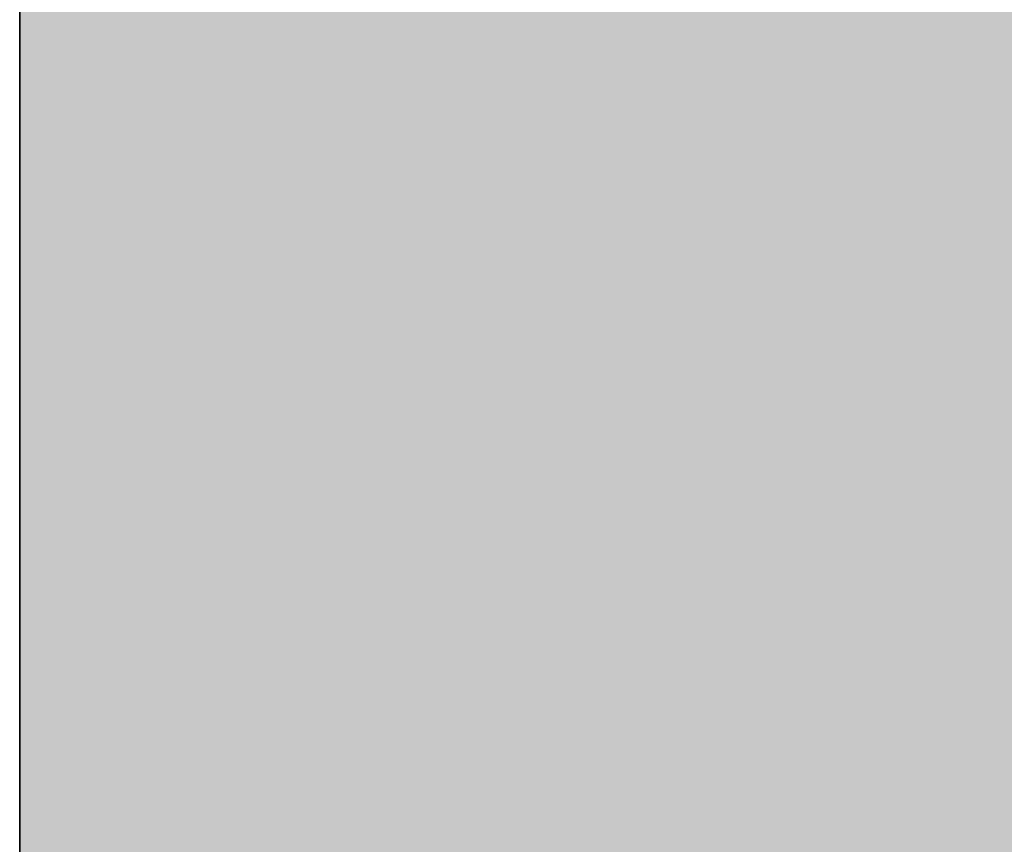
# Model space of a CAD drawing. Units: inches. Extents: x 2091 to 2899, y 967 to 2217.
# Tile 172 of 256: x 2203.143603 to 2203.151632, y 1152.253784 to 1152.260509. Entities that reach past the tile are written whole.
import ezdxf

# ---------------------------------------------------------------- set-up
doc = ezdxf.new("R2010")
doc.units = ezdxf.units.IN
doc.layers.add('A-WALL-PATT', color=141, linetype='Continuous', lineweight=13, true_color=0xadddf7)
doc.layers.add('C-PROP', color=7, linetype='Continuous', lineweight=35)

msp = doc.modelspace()

# ---------------------------------------------------------------- hatches: boundary and pattern name
at = {"layer": 'A-WALL-PATT'}
h = msp.add_hatch(color=256, dxfattribs=at)
h.dxf.hatch_style = 1
h.paths.add_polyline_path([(2803.1436027, 2050.9190588), (2203.1436027, 2050.9190588), (2203.1436027, 1090.9190588), (2803.1436027, 1090.9190588)])
h.paths.add_polyline_path([(2635.7988501, 1147.5404649), (2674.5240524, 1147.5404649, 0.376086), (2678.5296653, 1152.8802017), (2678.5296653, 1159.5564734, 0.333335), (2674.524319, 1163.561846), (2674.524319, 1163.5618504), (2674.524319, 1192.9343904), (2635.8059707, 1192.9343904), (2597.0876225, 1192.9343904), (2597.0876225, 1163.561846, 0.333335), (2593.0822761, 1159.5564734), (2593.0822761, 1152.8802017, 0.376086), (2597.087889, 1147.5404649)], flags=0)
h.paths.add_polyline_path([(2436.0104329, 1278.2407784, 0.000483), (2435.9526433, 1278.215027, -0.001328), (2435.9356253, 1278.1116934, -0.001711), (2436.1164401, 1278.0407583, 0.002185)], flags=0)
h.paths.add_polyline_path([(2794.1436027, 1143.4190588), (2794.1436027, 1347.4190588), (2543.3701706, 1347.4190588), (2543.3701706, 1351.9190588), (2794.1436027, 1351.9190588), (2794.1436027, 1392.7135549), (2793.9473982, 1392.7135549), (2793.9473982, 1473.5368999), (2794.1436027, 1473.5368999), (2794.1436027, 1531.9190588), (2650.1436027, 1531.9190588), (2650.1436027, 1536.4190588), (2794.1436027, 1536.4190588), (2794.1436027, 1692.4190588), (2609.3756095, 1692.4190588), (2609.3756095, 1644.4190588), (2604.8756095, 1644.4190588), (2604.8756095, 1744.9190588), (2609.3756095, 1744.9190588), (2609.3756095, 1696.9190588), (2794.1436027, 1696.9190588), (2794.1436027, 1780.9190588), (2609.6436027, 1780.9190588), (2493.8756095, 1780.9190588), (2493.8756095, 1785.4190588), (2609.6436027, 1785.4190588), (2794.1436027, 1785.4190588), (2794.1436027, 1847.9388214), (2793.9512217, 1847.9388214), (2793.9512217, 1928.7621663), (2794.1436027, 1928.7621663), (2794.1436027, 1941.4190588), (2614.1436027, 1941.4190588), (2614.1436027, 1821.4190588), (2609.6436027, 1821.4190588), (2609.6436027, 1941.4190588), (2392.1436027, 1941.4190588), (2392.1436027, 1819.9190588), (2387.6436027, 1819.9190588), (2387.6436027, 1941.4190588), (2212.1436027, 1941.4190588), (2212.1436027, 1783.9190588), (2392.1436027, 1783.9190588), (2392.1436027, 1780.9190588), (2212.1436027, 1780.9190588), (2212.1436027, 1629.4190588), (2387.6436027, 1629.4190588), (2387.6436027, 1744.9190588), (2392.1436027, 1744.9190588), (2392.1436027, 1627.9190588), (2317.1436027, 1627.9190588), (2317.1436027, 1551.4190588), (2317.1436027, 1536.4190588), (2459.3835909, 1536.4190588), (2459.3835909, 1602.3964802), (2463.8835909, 1602.3964802), (2463.8835909, 1531.9190588), (2456.6436027, 1531.9190588), (2456.6436027, 1529.9190588), (2452.1436027, 1529.9190588), (2452.1436027, 1531.9190588), (2312.6436027, 1531.9190588), (2312.6436027, 1551.4190588), (2306.1436027, 1551.4190588), (2306.1436027, 1555.9190588), (2308.1436027, 1555.9190588), (2308.1436027, 1551.4190588), (2312.6436027, 1551.4190588), (2312.6436027, 1627.9190588), (2212.1436027, 1627.9190588), (2212.1436027, 1555.9190588), (2270.1436027, 1555.9190588), (2270.1436027, 1551.4190588), (2212.1436027, 1551.4190588), (2212.1436027, 1351.9190588), (2272.1436027, 1351.9190588), (2272.1436027, 1347.4190588), (2212.1436027, 1347.4190588), (2212.1436027, 1275.4190588), (2308.1436027, 1275.4190588), (2308.1436027, 1351.9190588), (2452.1436027, 1351.9190588), (2452.1436027, 1493.9190588), (2456.6436027, 1493.9190588), (2456.6436027, 1347.4190588), (2312.6436027, 1347.4190588), (2312.6436027, 1270.9190588), (2212.1436027, 1270.9190588), (2212.1436027, 1099.9190588), (2281.2375229, 1099.9190588), (2282.8710413, 1110.9138034), (2282.0083413, 1116.9966034), (2278.5577413, 1121.4204034), (2268.2056413, 1128.0562034), (2272.0876413, 1128.0562034), (2273.8129413, 1131.9270034), (2279.4203413, 1134.6919034), (2285.0278413, 1135.2449034), (2287.6158413, 1137.4568034), (2288.0471413, 1138.0098034), (2289.3411413, 1140.7747034), (2291.0665413, 1139.6687034), (2292.3605413, 1135.2449034), (2295.3798413, 1136.9038034), (2296.2425413, 1135.7979034), (2297.1052413, 1133.0330034), (2300.1246413, 1138.0098034), (2303.1439413, 1138.0098034), (2304.4379413, 1135.7979034), (2303.1439413, 1133.5860034), (2306.5946413, 1134.6919034), (2307.8887413, 1133.0330034), (2310.9080413, 1135.2449034), (2313.9274413, 1134.1389034), (2315.6268599, 1132.4271023), (2308.3200413, 1117.5496034), (2290.2038413, 1109.8079034), (2288.9098413, 1103.1721034), (2289.2723086, 1099.9190588), (2434.9182274, 1099.9190588), (2431.5932274, 1124.7880588), (2429.9302274, 1169.5530588), (2430.9271848, 1240.5196942), (2435.6589255, 1238.1861258), (2437.1352274, 1196.5540588), (2438.7982274, 1143.9730588), (2442.6782274, 1111.9980588), (2446.5582274, 1099.9190588), (2794.1436027, 1099.9190588), (2794.1436027, 1138.9190588), (2548.0324471, 1138.9190588), (2548.0324471, 1143.4190588), (2548.0324471, 1148.8190588), (2546.6684571, 1148.0315588), (2528.6856919, 1179.1786218, 0.256256), (2512.0324471, 1148.8190588), (2512.0324471, 1143.4190588), (2512.0324471, 1138.9190588), (2507.5324471, 1138.9190588), (2507.5324471, 1143.4190588), (2507.5324471, 1148.8190588, 0.256256), (2490.8792023, 1179.1786218), (2472.8964371, 1148.0315588), (2471.5324471, 1148.8190588), (2471.5324471, 1143.4190588), (2467.0324471, 1143.4190588), (2467.0324471, 1269.9457858, 0.039061), (2460.9099871, 1273.5800588), (2467.0324471, 1273.5800588), (2467.0324471, 1286.3253638, 0.014511), (2465.2161944, 1286.7619052), (2467.0324471, 1287.0525761), (2467.0324471, 1323.4190588), (2471.5324471, 1323.4190588), (2471.5324471, 1148.8190588), (2489.5324471, 1179.9959734), (2490.8964371, 1179.2084734), (2490.8792023, 1179.1786218, -0.256256), (2507.5324471, 1148.8190588), (2507.5324471, 1143.4190588), (2512.0324471, 1143.4190588), (2512.0324471, 1148.8190588, -0.256256), (2528.6856919, 1179.1786218), (2528.6684571, 1179.2084734), (2530.0324471, 1179.9959734), (2548.0324471, 1148.8190588), (2548.0324471, 1143.4190588)], flags=16)
h.paths.add_polyline_path([(2607.7685461, 1200.9450832), (2607.7685461, 1265.0306251), (2597.0876225, 1281.0520106), (2619.7845852, 1281.0520106), (2627.795278, 1337.1268598), (2635.7988501, 1337.1268598), (2643.8166634, 1337.1268598), (2651.8273562, 1281.0520106), (2674.524319, 1281.0520106), (2663.8433953, 1265.0306251), (2663.8433953, 1200.9450832), (2635.8059707, 1200.9450832)], flags=0)
edge = h.paths.add_edge_path(flags=0)
edge.add_ellipse((13303.8962153, 1272.9987247), major_axis=(-10595.3130399, 0.0000005), ratio=0.842303870086, start_angle=0.62823721906, end_angle=0.64655409989, ccw=False)
edge.add_ellipse((2711.7004495, 1156.8526781), major_axis=(2.2197691, 0), ratio=0.84230387, start_angle=111.5352435, end_angle=180.6282372, ccw=False)
edge.add_ellipse((13303.1562922, 1272.9987246), major_axis=(-10593.0263064, 0), ratio=0.842303869544, start_angle=0.52827147182, end_angle=0.64655409706, ccw=False)
edge.add_line((2710.7645961, 1175.3332951), (2710.1299858, 1175.3332951))
edge.add_ellipse((2710.1299858, 1176.5797752), major_axis=(1.4798461, 0), ratio=0.84230387, start_angle=180, end_angle=270, ccw=False)
edge.add_line((2708.6501397, 1176.5797752), (2708.6501397, 1200.7829144))
edge.add_ellipse((2710.1299858, 1200.7829144), major_axis=(1.4798461, 0), ratio=0.84230387, start_angle=90, end_angle=180, ccw=False)
edge.add_line((2710.1299858, 1202.0293944), (2710.4650752, 1202.0293944))
edge.add_ellipse((13303.1562922, 1272.9987246), major_axis=(-10593.0263064, 0), ratio=0.842303869544, start_angle=-0.09022908859, end_angle=0.38386677879, ccw=False)
edge.add_ellipse((2710.1299858, 1290.9270308), major_axis=(-1.4798461, 0), ratio=0.84230387, start_angle=0, end_angle=90, ccw=False)
edge.add_line((2708.6501397, 1290.9270308), (2708.6501397, 1315.13017))
edge.add_ellipse((2710.1299858, 1315.13017), major_axis=(-1.4798461, 0), ratio=0.84230387, start_angle=-90, end_angle=0, ccw=False)
edge.add_line((2710.1299858, 1316.3766501), (2710.7063141, 1316.3766501))
edge.add_ellipse((3238.4017202, 1296.2895655), major_axis=(528.2339998, 0), ratio=0.84230386954, start_angle=176.349572414, end_angle=177.820049686, ccw=False)
edge.add_ellipse((2775.0630432, 1071.4506962), major_axis=(313.3077613, 0), ratio=0.84230386954, start_angle=102.125965552, end_angle=103.780528989, ccw=False)
edge.add_ellipse((2775.0630432, 1078.3056979), major_axis=(-305.3028915, 0), ratio=0.84230386955, start_angle=-79.790461003, end_angle=-77.555372706, ccw=False)
edge.add_ellipse((2695.1417666, 1541.9753825), major_axis=(-250.9602162, 0), ratio=0.84230386954, start_angle=99.256566007, end_angle=102.554932644)
edge.add_line((2741.4103262, 1334.2142554), (2747.1325454, 1337.3784768))
edge.add_ellipse((2747.5386163, 1336.8574776), major_axis=(-0.739923, 0), ratio=0.84230387, start_angle=270, end_angle=307.9331305, ccw=False)
edge.add_ellipse((2747.5386163, 1336.8574776), major_axis=(-0.739923, 0), ratio=0.84230387, start_angle=232.0668695, end_angle=270, ccw=False)
edge.add_line((2747.9446872, 1337.3784768), (2753.6669064, 1334.2142554))
edge.add_ellipse((2799.935466, 1541.9753825), major_axis=(250.9602162, 0), ratio=0.84230386954, start_angle=257.445067356, end_angle=260.743433993)
edge.add_ellipse((2720.0141894, 1078.3056979), major_axis=(305.3028915, 0), ratio=0.84230386954, start_angle=77.555372707, end_angle=79.790461003, ccw=False)
edge.add_ellipse((2720.0141894, 1071.4506962), major_axis=(-313.3077613, 0), ratio=0.84230386954, start_angle=256.219471011, end_angle=257.874034448, ccw=False)
edge.add_ellipse((2256.6755124, 1296.2895655), major_axis=(-528.2339998, 0), ratio=0.84230386954, start_angle=182.179950314, end_angle=183.650427586, ccw=False)
edge.add_line((2784.3709184, 1316.3766501), (2784.9472468, 1316.3766501))
edge.add_ellipse((2784.9472468, 1315.13017), major_axis=(1.4798461, 0), ratio=0.84230387, start_angle=0, end_angle=90, ccw=False)
edge.add_line((2786.4270928, 1315.13017), (2786.4270928, 1290.9270308))
edge.add_ellipse((2784.9472468, 1290.9270308), major_axis=(1.4798461, 0), ratio=0.84230387, start_angle=270, end_angle=360, ccw=False)
edge.add_ellipse((-7808.0790596, 1272.9987246), major_axis=(10593.0263063, 0), ratio=0.842303869544, start_angle=-0.38386677879, end_angle=0.09022908859, ccw=False)
edge.add_line((2784.6121574, 1202.0293944), (2784.9472468, 1202.0293944))
edge.add_ellipse((2784.9472468, 1200.7829144), major_axis=(1.4798461, 0), ratio=0.84230387, start_angle=0, end_angle=90, ccw=False)
edge.add_line((2786.4270928, 1200.7829144), (2786.4270928, 1176.5797752))
edge.add_ellipse((2784.9472468, 1176.5797752), major_axis=(-1.4798461, 0), ratio=0.84230387, start_angle=90, end_angle=180, ccw=False)
edge.add_line((2784.9472468, 1175.3332951), (2784.3126365, 1175.3332951))
edge.add_ellipse((-7808.0790596, 1272.9987246), major_axis=(10593.0263063, 0), ratio=0.842303869544, start_angle=-0.61864319632, end_angle=-0.52827147182, ccw=False)
edge.add_ellipse((2783.3767831, 1156.8526781), major_axis=(-2.2197691, 0), ratio=0.84230387, start_angle=179.3717628, end_angle=248.4647566, ccw=False)
edge.add_ellipse((-7808.8189826, 1272.9987246), major_axis=(-10595.3130398, 0.0000036), ratio=0.842303865762, start_angle=179.3534459226, end_angle=179.37176280343, ccw=False)
edge.add_ellipse((2780.2973026, 1153.500793), major_axis=(-5.2464256, 0), ratio=0.84230387, start_angle=90, end_angle=179.3534459, ccw=False)
edge.add_line((2780.2973026, 1149.0817084), (2714.77993, 1149.0817084))
edge.add_ellipse((2714.77993, 1153.500793), major_axis=(5.2464256, 0), ratio=0.84230387, start_angle=180.6465541, end_angle=270, ccw=False)
edge = h.paths.add_edge_path(flags=0)
edge.add_line((2718.1873674, 1151.0078329), (2718.1873674, 1170.4723638))
edge.add_ellipse((2721.1470595, 1170.4723638), major_axis=(-2.9596921, 0), ratio=0.84230387, start_angle=-90, end_angle=0, ccw=False)
edge.add_line((2721.1470595, 1172.965324), (2773.9301731, 1172.965324))
edge.add_ellipse((2773.9301731, 1170.4723638), major_axis=(-2.9596921, 0), ratio=0.84230387, start_angle=180, end_angle=270, ccw=False)
edge.add_line((2776.8898652, 1170.4723638), (2776.8898652, 1151.0078329))
edge.add_line((2776.8898652, 1151.0078329), (2718.1873674, 1151.0078329))
edge = h.paths.add_edge_path(flags=0)
edge.add_line((2718.1873674, 1180.2341502), (2718.1873674, 1199.0578342))
edge.add_ellipse((2747.5386163, 1320.3986402), major_axis=(147.0179239, 0), ratio=0.84230386954, start_angle=256.40186531, end_angle=283.59813469)
edge.add_line((2776.8898652, 1199.0578342), (2776.8898652, 1180.2341502))
edge.add_ellipse((2747.5386163, 1301.5749562), major_axis=(147.0179239, 0), ratio=0.84230386954, start_angle=256.40186531, end_angle=283.59813469, ccw=False)
edge = h.paths.add_edge_path(flags=0)
edge.add_ellipse((13303.1562922, 1272.9987246), major_axis=(-10591.5464603, 0), ratio=0.842303869555, start_angle=0.05559431352, end_angle=0.37776419393, ccw=False)
edge.add_line((2711.6168595, 1262.7217103), (2715.6674076, 1249.4953957))
edge.add_ellipse((6413.8919626, 1241.691919), major_axis=(-3698.2361592, 0), ratio=0.842303869547, start_angle=-0.120897369, end_angle=0.3640763489)
edge.add_line((2715.7610383, 1218.1924547), (2711.9343065, 1203.167361))
edge = h.paths.add_edge_path(flags=0)
edge.add_line((2718.1873674, 1251.074566), (2716.0024854, 1267.4504351))
edge.add_ellipse((2742.1511746, 1202.1895399), major_axis=(81.7725845, 0), ratio=0.8423038695, start_angle=94.277420963, end_angle=111.834953797, ccw=False)
edge.add_line((2737.0097482, 1270.9306255), (2758.0674844, 1270.9306255))
edge.add_ellipse((2752.926058, 1202.1895399), major_axis=(81.7725845, 0), ratio=0.8423038695, start_angle=68.165046203, end_angle=85.722579037, ccw=False)
edge.add_line((2779.0747472, 1267.4504351), (2776.8898652, 1251.074566))
edge.add_ellipse((2750.3380588, 1187.8853558), major_axis=(79.5796641, 0), ratio=0.8423038695, start_angle=67.208085122, end_angle=85.129930403)
edge.add_line((2756.0346562, 1254.7436557), (2739.0425764, 1254.7436557))
edge.add_ellipse((2744.7391738, 1187.8853558), major_axis=(79.5796641, 0), ratio=0.8423038695, start_angle=94.870069597, end_angle=112.791914878)
edge = h.paths.add_edge_path(flags=0)
edge.add_line((2783.1429261, 1203.167361), (2779.3161943, 1218.1924547))
edge.add_ellipse((-918.81473, 1241.691919), major_axis=(3698.2361592, 0), ratio=0.842303869546, start_angle=-0.3640763489, end_angle=0.120897369)
edge.add_line((2779.409825, 1249.4953957), (2783.4603731, 1262.7217103))
edge.add_ellipse((-7808.0790596, 1272.9987246), major_axis=(-10591.5464603, 0), ratio=0.84230386954, start_angle=179.6222358061, end_angle=179.94440568651, ccw=False)
edge = h.paths.add_edge_path(flags=0)
edge.add_ellipse((2734.2008921, 1286.6904402), major_axis=(-0.3566086, 6.3400775), ratio=0.603833576, start_angle=89.00201428, end_angle=253.65740805, ccw=False)
edge.add_line((2730.3690013, 1286.5418057), (2730.3690013, 1301.3519803))
edge.add_line((2730.3690013, 1301.3519803), (2735.9133107, 1305.2148028))
edge.add_ellipse((2736.3849168, 1304.7345612), major_axis=(0.739923, 0), ratio=0.84230387, start_angle=90, end_angle=134.4802109, ccw=False)
edge.add_line((2736.3849168, 1305.3578013), (2738.0327829, 1305.3578013))
edge.add_line((2738.0327829, 1305.3578013), (2738.0327829, 1307.7079274))
edge.add_ellipse((2794.201642, 1307.7079274), major_axis=(56.168859, 0), ratio=0.8423038695, start_angle=150.5614304, end_angle=180, ccw=False)
edge.add_ellipse((2700.8755906, 1307.7079274), major_axis=(-56.168859, 0), ratio=0.8423038695, start_angle=180, end_angle=209.4385696, ccw=False)
edge.add_line((2757.0444497, 1307.7079274), (2757.0444497, 1305.3578013))
edge.add_line((2757.0444497, 1305.3578013), (2758.6923157, 1305.3578013))
edge.add_ellipse((2758.6923157, 1304.7345612), major_axis=(-0.739923, 0), ratio=0.84230387, start_angle=225.5197891, end_angle=270, ccw=False)
edge.add_line((2759.1639219, 1305.2148028), (2764.7082312, 1301.3519803))
edge.add_line((2764.7082312, 1301.3519803), (2764.7082312, 1286.5418057))
edge.add_ellipse((2760.8763405, 1286.6904402), major_axis=(0.3566086, 6.3400775), ratio=0.603833576, start_angle=106.34259195, end_angle=270.99798572, ccw=False)
edge.add_line((2757.0444497, 1285.7970896), (2757.0444497, 1307.7079274))
edge.add_ellipse((2700.8755906, 1307.7079274), major_axis=(-56.168859, 0), ratio=0.8423038695, start_angle=180, end_angle=209.4385696)
edge.add_ellipse((2794.201642, 1307.7079274), major_axis=(56.168859, 0), ratio=0.8423038695, start_angle=150.5614304, end_angle=180)
edge.add_line((2738.0327829, 1307.7079274), (2738.0327829, 1285.7970896))
h.paths.add_polyline_path([(2417.8122727, 1104.449704), (2413.4922727, 1102.529704), (2410.6122727, 1103.969704), (2409.1722727, 1106.369704), (2407.2522727, 1107.329704), (2406.2922727, 1109.729704), (2405.3322727, 1114.049704), (2405.3322727, 1117.889704), (2406.2922727, 1120.129704), (2407.2522727, 1119.809704), (2408.8483218, 1118.3276585), (2410.1739451, 1119.4241703), (2410.2112727, 1120.405704), (2411.0407305, 1121.4190541), (2410.6992727, 1119.858704), (2410.1739451, 1119.4241703), (2410.0884515, 1117.1761095), (2411.1328361, 1116.2063237), (2413.9722727, 1119.329704), (2416.8522727, 1120.769704), (2416.8697209, 1120.7987842), (2417.0350713, 1119.4051162), (2417.8962134, 1118.1433844), (2418.2922727, 1118.369704), (2419.5444467, 1120.0392692), (2419.3609153, 1118.387487), (2419.0321078, 1119.3561507), (2418.3989394, 1118.5119262), (2419.2522727, 1114.529704), (2418.7940909, 1107.1987949)], flags=0)
h.paths.add_polyline_path([(2508.8701706, 1347.4190588), (2508.3701706, 1347.4190588), (2508.3701706, 1351.9190588), (2508.8701706, 1351.9190588)], flags=0)
h.paths.add_polyline_path([(2473.3701706, 1347.4190588), (2472.3701706, 1347.4190588), (2467.8701706, 1347.4190588), (2467.8701706, 1455.4190588), (2472.3701706, 1455.4190588), (2472.3701706, 1352.4190588), (2473.3701706, 1352.4190588)], flags=0)
h.paths.add_polyline_path([(2352.106244, 1217.4461971), (2349.226244, 1218.8861971), (2347.786244, 1221.2861971), (2345.866244, 1222.2461971), (2344.906244, 1224.6461971), (2343.946244, 1228.9661971), (2343.946244, 1232.8061971), (2344.906244, 1235.0461971), (2345.866244, 1234.7261971), (2347.4622931, 1233.2441515), (2348.7879164, 1234.3406634), (2348.825244, 1235.3221971), (2349.6547018, 1236.3355471), (2349.313244, 1234.7751971), (2348.7879164, 1234.3406634), (2348.7024228, 1232.0926025), (2349.7468074, 1231.1228168), (2352.586244, 1234.2461971), (2355.466244, 1235.6861971), (2355.4836921, 1235.7152773), (2355.6490426, 1234.3216093), (2356.5101846, 1233.0598774), (2356.906244, 1233.2861971), (2358.1584179, 1234.9557623), (2357.9748866, 1233.3039801), (2357.6460791, 1234.2726438), (2357.0129107, 1233.4284193), (2357.866244, 1229.4461971), (2357.4080622, 1222.115288), (2356.426244, 1219.3661971)], flags=0)
h.paths.add_polyline_path([(2348.2967999, 1112.2244204), (2347.0137999, 1112.3104204), (2345.5297999, 1114.1274204), (2345.7317999, 1115.8584204), (2346.8117999, 1116.9824204), (2346.8117999, 1114.6464204), (2345.8667999, 1114.2144204), (2346.8797999, 1114.3004204)], flags=0)
h.paths.add_polyline_path([(2347.0137999, 1110.9264204), (2346.2717999, 1110.4934204), (2346.6097999, 1111.1864204)], flags=0)
h.paths.add_polyline_path([(2345.8667999, 1118.1944204), (2345.5297999, 1117.3294204), (2343.7077999, 1118.0214204), (2344.3827999, 1118.6264204)], flags=0)
h.paths.add_polyline_path([(2346.6767999, 1109.2824204), (2346.0697999, 1108.0714204), (2345.8667999, 1110.0614204)], flags=0)
h.paths.add_polyline_path([(2345.0567999, 1119.7514204), (2343.6397999, 1119.7514204), (2343.9777999, 1121.1354204)], flags=0)
h.paths.add_polyline_path([(2345.2597999, 1116.5504204), (2345.1247999, 1115.8584204), (2344.9217999, 1115.6854204), (2344.7197999, 1116.3774204)], flags=0)
h.paths.add_polyline_path([(2345.6647999, 1112.3104204), (2345.4617999, 1111.5324204), (2344.0447999, 1111.9644204), (2344.6517999, 1112.5704204)], flags=0)
h.paths.add_polyline_path([(2345.1917999, 1113.3494204), (2344.4497999, 1113.8684204), (2344.7197999, 1114.3874204)], flags=0)
h.paths.add_polyline_path([(2344.6517999, 1116.8094204), (2344.1797999, 1115.6854204), (2344.6517999, 1115.3394204), (2343.9097999, 1114.9064204), (2343.0327999, 1115.9444204), (2343.6397999, 1116.4634204)], flags=0)
h.paths.add_polyline_path([(2345.8667999, 1106.6864204), (2344.9897999, 1105.5624204), (2344.5167999, 1106.6004204)], flags=0)
h.paths.add_polyline_path([(2344.8547999, 1110.0614204), (2344.5167999, 1109.2824204), (2344.1127999, 1109.7154204)], flags=0)
h.paths.add_polyline_path([(2344.0447999, 1113.5224204), (2343.4377999, 1113.0894204), (2342.7627999, 1113.9544204)], flags=0)
h.paths.add_polyline_path([(2344.3147999, 1111.0124204), (2342.9647999, 1110.3204204), (2342.9647999, 1111.0994204)], flags=0)
h.paths.add_polyline_path([(2345.1247999, 1104.6974204), (2344.5847999, 1103.7454204), (2344.4497999, 1104.2644204)], flags=0)
h.paths.add_polyline_path([(2342.8297999, 1121.2224204), (2341.7497999, 1120.5304204), (2340.5357999, 1121.0494204), (2340.1307999, 1121.8284204), (2340.6707999, 1122.9524204), (2341.1427999, 1121.8284204), (2341.6147999, 1122.0014204)], flags=0)
h.paths.add_polyline_path([(2342.9647999, 1119.7514204), (2343.0327999, 1118.4534204), (2342.0877999, 1118.0214204), (2342.0197999, 1119.4914204)], flags=0)
h.paths.add_polyline_path([(2342.6947999, 1116.8964204), (2341.9527999, 1116.6364204), (2342.0197999, 1117.3294204)], flags=0)
h.paths.add_polyline_path([(2343.0327999, 1112.2244204), (2342.0197999, 1111.7914204), (2341.5477999, 1112.2244204), (2342.3577999, 1113.3494204)], flags=0)
h.paths.add_polyline_path([(2343.7747999, 1104.4374204), (2342.6277999, 1102.8804204), (2342.6947999, 1104.6104204), (2343.4377999, 1105.1294204)], flags=0)
h.paths.add_polyline_path([(2342.0197999, 1115.0794204), (2340.8057999, 1115.5124204), (2340.9407999, 1116.3774204)], flags=0)
h.paths.add_polyline_path([(2341.4807999, 1120.0974204), (2341.4807999, 1119.4054204), (2341.0757999, 1119.5784204), (2341.1427999, 1120.0974204)], flags=0)
h.paths.add_polyline_path([(2341.8177999, 1114.4734204), (2340.9407999, 1113.0894204), (2340.8057999, 1114.5604204)], flags=0)
h.paths.add_polyline_path([(2341.1427999, 1118.5404204), (2340.9407999, 1116.9824204), (2339.0507999, 1117.6754204), (2339.0507999, 1118.6264204)], flags=0)
h.paths.add_polyline_path([(2342.6947999, 1101.6684204), (2341.9527999, 1101.8414204), (2342.5597999, 1102.3614204)], flags=0)
h.paths.add_polyline_path([(2340.3327999, 1119.6654204), (2338.4437999, 1119.5784204), (2337.9037999, 1120.3574204), (2339.6577999, 1120.6164204)], flags=0)
h.paths.add_polyline_path([(2340.3327999, 1115.3394204), (2340.0627999, 1113.6954204), (2339.3877999, 1115.3394204)], flags=0)
h.paths.add_polyline_path([(2341.8177999, 1103.8314204), (2341.5477999, 1102.8804204), (2341.1427999, 1103.6584204)], flags=0)
h.paths.add_polyline_path([(2339.0507999, 1122.8664204), (2337.2957999, 1121.8284204), (2337.0937999, 1123.1254204), (2337.7687999, 1123.8184204)], flags=0)
h.paths.add_polyline_path([(2339.1177999, 1121.7414204), (2338.8477999, 1121.2224204), (2338.1737999, 1121.0494204), (2338.3757999, 1121.5684204)], flags=0)
h.paths.add_polyline_path([(2339.1857999, 1119.3194204), (2338.6457999, 1118.7134204), (2338.2407999, 1118.1074204), (2338.2407999, 1118.8864204)], flags=0)
h.paths.add_polyline_path([(2341.1427999, 1101.9284204), (2340.6027999, 1101.2364204), (2340.0627999, 1101.8414204), (2340.6027999, 1102.3614204)], flags=0)
h.paths.add_polyline_path([(2337.6337999, 1117.7614204), (2336.6207999, 1118.2804204), (2337.2957999, 1118.9724204)], flags=0)
h.paths.add_polyline_path([(2336.8237999, 1119.5784204), (2334.7987999, 1118.9724204), (2335.2037999, 1120.3574204), (2336.5537999, 1120.8764204)], flags=0)
h.paths.add_polyline_path([(2339.1177999, 1100.4574204), (2337.3637999, 1100.5434204), (2336.7557999, 1101.2364204)], flags=0)
h.paths.add_polyline_path([(2336.3507999, 1122.4334204), (2336.0137999, 1121.9144204), (2334.9337999, 1122.4334204), (2334.5287999, 1123.4714204), (2335.7437999, 1122.7794204)], flags=0)
h.paths.add_polyline_path([(2334.7317999, 1120.8764204), (2334.2587999, 1120.3574204), (2334.0567999, 1120.7894204), (2334.5967999, 1121.3084204)], flags=0)
h.paths.add_polyline_path([(2334.4617999, 1122.1744204), (2332.5717999, 1121.3084204), (2331.3567999, 1122.1744204), (2332.0997999, 1122.8664204)], flags=0)
h.paths.add_polyline_path([(2334.2587999, 1118.5404204), (2333.3817999, 1118.4534204), (2333.6517999, 1119.3194204)], flags=0)
h.paths.add_polyline_path([(2335.5417999, 1102.2744204), (2334.1917999, 1102.6204204), (2335.2717999, 1103.3124204)], flags=0)
h.paths.add_polyline_path([(2332.7067999, 1119.6654204), (2331.6947999, 1120.4434204), (2332.5047999, 1120.7894204)], flags=0)
h.paths.add_polyline_path([(2334.7317999, 1101.1494204), (2333.5167999, 1101.5824204), (2333.9887999, 1101.7554204)], flags=0)
h.paths.add_polyline_path([(2332.6397999, 1116.6364204), (2331.0867999, 1116.2904204), (2331.9647999, 1118.1944204)], flags=0)
h.paths.add_polyline_path([(2330.7497999, 1121.5684204), (2330.2767999, 1120.2704204), (2328.5227999, 1119.3194204), (2328.9947999, 1121.0494204)], flags=0)
h.paths.add_polyline_path([(2330.7497999, 1118.6264204), (2330.0077999, 1117.5024204), (2329.8727999, 1118.0214204)], flags=0)
h.paths.add_polyline_path([(2332.0997999, 1102.3614204), (2330.5467999, 1102.0144204), (2331.6947999, 1102.9664204)], flags=0)
h.paths.add_polyline_path([(2329.5347999, 1113.6084204), (2329.0627999, 1112.3104204), (2328.5897999, 1113.3494204)], flags=0)
h.paths.add_polyline_path([(2328.3877999, 1117.8484204), (2327.5097999, 1116.5504204), (2327.1727999, 1117.7614204)], flags=0)
h.paths.add_polyline_path([(2329.7377999, 1106.5134204), (2329.5347999, 1105.3024204), (2328.2527999, 1106.0814204)], flags=0)
h.paths.add_polyline_path([(2328.6577999, 1114.3874204), (2328.0497999, 1114.1274204), (2328.3197999, 1114.9064204)], flags=0)
h.paths.add_polyline_path([(2328.3197999, 1112.2244204), (2327.1057999, 1112.1374204), (2326.7007999, 1112.6564204)], flags=0)
h.paths.add_polyline_path([(2326.9027999, 1115.2524204), (2326.7007999, 1114.1274204), (2325.2157999, 1113.6084204), (2326.0927999, 1115.3394204)], flags=0)
h.paths.add_polyline_path([(2326.6327999, 1108.3304204), (2326.0927999, 1107.3794204), (2325.8907999, 1108.5034204), (2326.4977999, 1109.1094204)], flags=0)
h.paths.add_polyline_path([(2615.1436027, 1531.9190588), (2609.6436027, 1531.9190588), (2609.6436027, 1620.4190588), (2614.1436027, 1620.4190588), (2614.1436027, 1536.4190588), (2615.1436027, 1536.4190588)], flags=0)
h.paths.add_polyline_path([(2545.1436027, 1563.4190588), (2464.1436027, 1563.4190588), (2464.1436027, 1632.4190588), (2509.1436027, 1632.4190588), (2509.1436027, 1627.9190588), (2509.1436027, 1603.9190588), (2468.6436027, 1603.9190588), (2468.6436027, 1567.9190588), (2540.6436027, 1567.9190588), (2540.6436027, 1591.9190588), (2545.1436027, 1591.9190588)], flags=0)
h.paths.add_polyline_path([(2388.9690483, 1549.985735), (2357.4341811, 1549.985735), (2357.4341811, 1623.3607783), (2399.3627772, 1623.3607783), (2435.6894654, 1623.3607783), (2435.5925469, 1602.5592734), (2435.5925469, 1602.3964802), (2388.9690483, 1602.3964802)], flags=0)
h.paths.add_polyline_path([(2388.8806282, 1555.8091511), (2374.9044295, 1555.8091511), (2374.9044295, 1600.5715641), (2374.9044295, 1615.4576454), (2406.3508766, 1615.4576454), (2406.3508766, 1618.9394309), (2412.1742927, 1615.4576454), (2406.3508766, 1611.9758599), (2406.3508766, 1615.4576454), (2388.8806282, 1615.4576454)], flags=0)
h.paths.add_polyline_path([(2568.8756095, 1644.4190588), (2453.3756095, 1644.4190588), (2453.3756095, 1785.4190588), (2457.8756095, 1785.4190588), (2457.8756095, 1648.9190588), (2568.8756095, 1648.9190588)], flags=0)
h.paths.add_polyline_path([(2212.1436027, 1945.9190588), (2212.1436027, 2041.9190588), (2794.1436027, 2041.9190588), (2794.1436027, 1945.9190588)], flags=16)
h.paths.add_polyline_path([(2271.0827276, 1964.3172377), (2776.852968, 1964.3172377), (2776.852968, 2037.1696226), (2271.0827276, 2037.1696226)], flags=8)
h.paths.add_polyline_path([(2380.6492852, 1536.8241435), (2461.0408087, 1536.8241435), (2461.0408087, 1554.6525871), (2380.6492852, 1554.6525871)], flags=8)
h.paths.add_polyline_path([(2240.7557092, 1609.7254508), (2309.1858294, 1609.7254508), (2309.1858294, 1617.6982037), (2240.7557092, 1617.6982037)], flags=8)
h.paths.add_polyline_path([(2212.6772554, 1313.5041021), (2282.5915203, 1313.5041021), (2282.5915203, 1322.7452389), (2212.6772554, 1322.7452389)], flags=8)
h.paths.add_polyline_path([(2457.111976, 1114.778574), (2558.4815807, 1114.778574), (2558.4815807, 1142.2196823), (2457.111976, 1142.2196823)], flags=8)
h.paths.add_polyline_path([(2473.4423372, 1273.0100672), (2604.6412257, 1273.0100672), (2604.6412257, 1318.3469349), (2473.4423372, 1318.3469349)], flags=8)
h.paths.add_polyline_path([(2638.8763024, 1626.9774316), (2684.2503675, 1627.9767377), (2684.0384825, 1637.5974944), (2638.6644174, 1636.5981884)], flags=8)
h.paths.add_polyline_path([(2537.5905538, 1453.7934466), (2628.3895472, 1453.7934466), (2628.3895472, 1475.3448114), (2537.5905538, 1475.3448114)], flags=8)
h.paths.add_polyline_path([(2504.1376376, 1714.6323972), (2554.6471875, 1714.6323972), (2554.6471875, 1730.2377115), (2504.1376376, 1730.2377115)], flags=8)
h.paths.add_polyline_path([(2487.5011806, 1575.6518716), (2535.0971214, 1575.6518716), (2535.0971214, 1598.3776456), (2487.5011806, 1598.3776456)], flags=8)
h.paths.add_polyline_path([(2709.0994004, 1735.7102784), (2740.0166009, 1735.7102784), (2740.0166009, 1749.9376406), (2709.0994004, 1749.9376406)], flags=8)
h.paths.add_polyline_path([(2442.4384239, 1792.1716575), (2564.7288353, 1792.1716575), (2564.7288353, 1842.0001626), (2442.4384239, 1842.0001626)], flags=8)
h.paths.add_polyline_path([(2655.8158012, 1809.6440763), (2789.5201425, 1806.6937963), (2790.0849768, 1832.2916379), (2656.3806355, 1835.2419179)], flags=8)
h.paths.add_polyline_path([(2234.8426972, 1797.7201432), (2368.5928512, 1794.7688523), (2369.1607182, 1820.504132), (2235.4105642, 1823.4554229)], flags=8)
h.paths.add_polyline_path([(2245.1384659, 1644.0063348), (2398.4277329, 1640.6238997), (2398.9948417, 1666.3248199), (2245.7055747, 1669.7072549)], flags=8)
h.paths.add_polyline_path([(2306.1428474, 1431.1685186), (2413.7683138, 1428.7936873), (2414.3331481, 1454.3915289), (2306.7076817, 1456.7663602)], flags=8)
h.paths.add_polyline_path([(2306.834582, 1458.2331447), (2393.3804836, 1456.3234487), (2393.9328082, 1481.3543583), (2307.3869066, 1483.2640542)], flags=8)

# ---------------------------------------------------------------- linework, layer by layer
at = {"layer": 'C-PROP'}
msp.add_lwpolyline([(2203.1436027, 2050.9190588), (2803.1436027, 2050.9190588), (2803.1436027, 1090.9190588), (2203.1436027, 1090.9190588)], close=True, dxfattribs=at)

doc.saveas('drawing.dxf')
